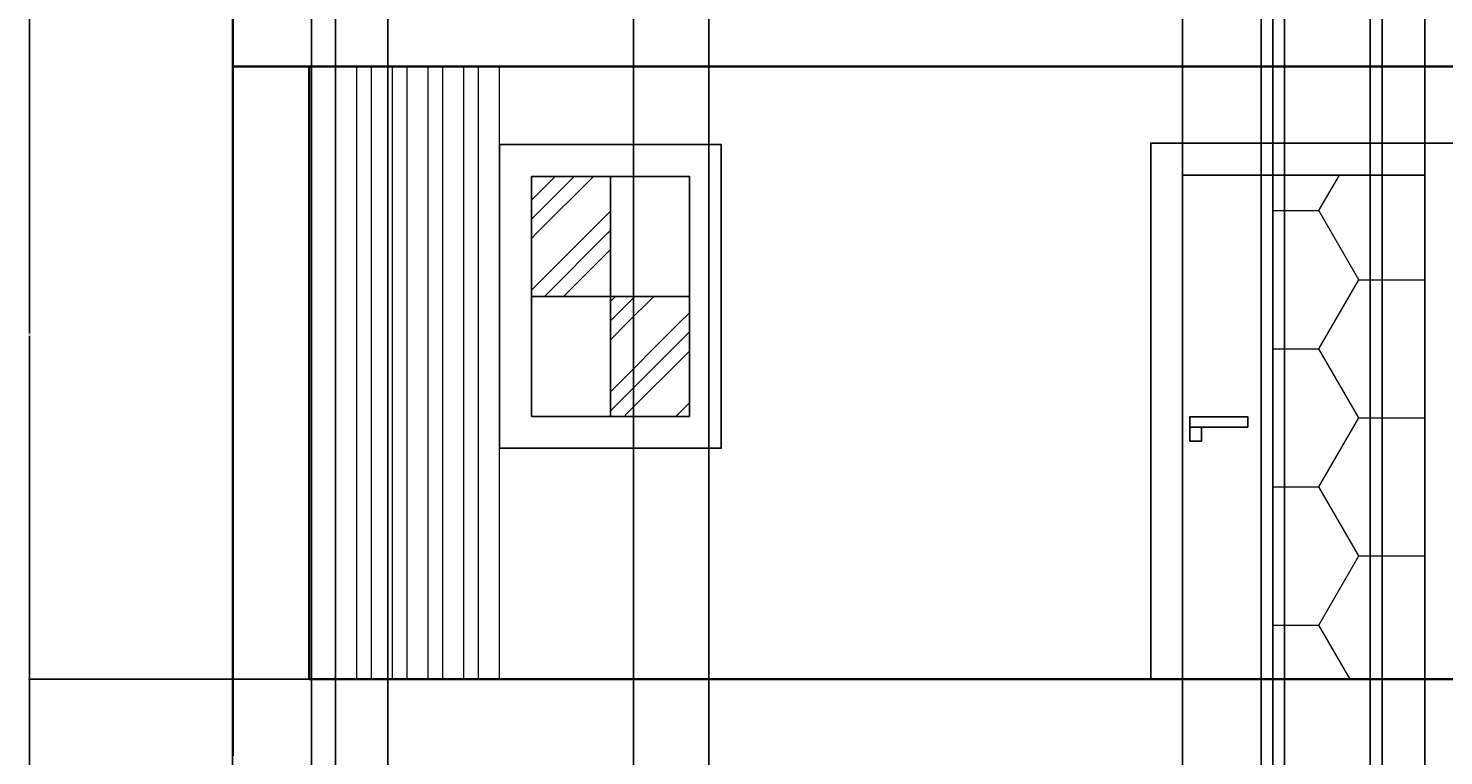
# Model space of a CAD drawing. Units: inches. Extents: x -8 to 554, y -200 to 499.
# Tile 2 of 12: x -8 to 214, y 7 to 121. Entities that reach past the tile are written whole.
import ezdxf

# ---------------------------------------------------------------- set-up
doc = ezdxf.new("R2010")
doc.units = ezdxf.units.IN
doc.header["$MEASUREMENT"] = 0
for name, color, linetype, lineweight in [('A-ANNO-DIMS', 2, 'Continuous', 18), ('A-DOOR', 3, 'Continuous', 25), ('A-DOOR-PATT', 252, 'Continuous', 13), ('A-FLOR', 7, 'Continuous', 35), ('A-GLAZ', 4, 'Continuous', 25), ('A-GLAZ-PATT', 252, 'Continuous', 13), ('A-WALL', 7, 'Continuous', 35), ('A-WALL-SCRN', 8, 'Continuous', 18)]:
    doc.layers.add(name, color=color, linetype=linetype, lineweight=lineweight)
doc.styles.get("Standard").update_dxf_attribs({"font": 'arial.ttf'})
doc.dimstyles.get("Standard").update_dxf_attribs({"dimtxt": 0.18, "dimasz": 0.18, "dimexe": 0.18, "dimexo": 0.0625, "dimgap": 0.09, "dimtad": 0, "dimtih": 1, "dimtoh": 1, "dimdec": 4, "dimzin": 0, "dimdsep": 46, "dimtxsty": 'Standard', "dimcen": 0.09, "dimadec": 0, "dimazin": 0, "dimtfac": 1, "dimtdec": 4, "dimtofl": 0, "dimtmove": 0, "dimatfit": 3, "dimfxl": 1, "dimtolj": 1, "dimtzin": 0, "dimarcsym": 0})

# ---------------------------------------------------------------- blocks, each defined once
blk = doc.blocks.new('DOOR-LEVER-ELEV')
for points in [[(0, 2.19), (9.08, 2.19), (9.08, 3.81), (0, 3.81)], [(0, 2.19), (1.8, 2.19), (1.8, 0), (0, 0)]]:
    blk.add_lwpolyline(points, close=True)
blk = doc.blocks.new('SCREEN-FIVE-FINS-ELEV')
for points in [[(0, 0), (3.37, 0), (3.37, 96), (0, 96)], [(5.59, 0), (8.97, 0), (8.97, 96), (5.59, 96)], [(11.19, 0), (14.56, 0), (14.56, 96), (11.19, 96)], [(16.78, 0), (20.16, 0), (20.16, 96), (16.78, 96)], [(22.38, 0), (25.75, 0), (25.75, 96), (22.38, 96)]]:
    blk.add_lwpolyline(points, close=True)
blk = doc.blocks.new('WINDOW-CASING-FOUR-LIGHT')
blk.add_lwpolyline([(0, 47.61), (34.77, 47.61), (34.77, 0), (0, 0)], close=True)
blk = doc.blocks.new('*D31')
at = {"layer": 'A-ANNO-DIMS', "color": 0, "lineweight": -2, "transparency": 16777216}
for p, q in [((24.34, 127.42), (24.34, -199.97)), ((453.32, -30.73), (453.32, -199.97)), ((24.52, -199.79), (238.54, -199.79)), ((453.14, -199.79), (239.12, -199.79))]:
    blk.add_line(p, q, dxfattribs=at)
at = {"layer": 'A-ANNO-DIMS', "color": 0, "transparency": 16777216}
for points in [[(24.52, -199.76), (24.52, -199.82), (24.34, -199.79)], [(453.14, -199.76), (453.14, -199.82), (453.32, -199.79)]]:
    blk.add_solid(points, dxfattribs=at)
at = {"layer": 'Defpoints', "color": 0, "transparency": 16777216}
for p in [(24.34, 127.48), (453.32, -30.67), (453.32, -199.79)]:
    blk.add_point(p, dxfattribs=at)
at = {"layer": 'A-ANNO-DIMS', "color": 0, "transparency": 16777216, "insert": (238.83, -199.79), "char_height": 0.18, "attachment_point": 5}
blk.add_mtext('\\A1;429', dxfattribs=at)
blk = doc.blocks.new('*D32')
at = {"layer": 'A-ANNO-DIMS', "color": 0, "lineweight": -2, "transparency": 16777216}
for p, q in [((24.34, 223.42), (24.34, -199.97)), ((444.34, 223.42), (444.34, -199.97)), ((24.52, -199.79), (234.05, -199.79)), ((444.16, -199.79), (234.63, -199.79))]:
    blk.add_line(p, q, dxfattribs=at)
at = {"layer": 'A-ANNO-DIMS', "color": 0, "transparency": 16777216}
for points in [[(24.52, -199.76), (24.52, -199.82), (24.34, -199.79)], [(444.16, -199.76), (444.16, -199.82), (444.34, -199.79)]]:
    blk.add_solid(points, dxfattribs=at)
at = {"layer": 'Defpoints', "color": 0, "transparency": 16777216}
for p in [(24.34, 223.48), (444.34, 223.48), (444.34, -199.79)]:
    blk.add_point(p, dxfattribs=at)
at = {"layer": 'A-ANNO-DIMS', "color": 0, "transparency": 16777216, "insert": (234.34, -199.79), "char_height": 0.18, "attachment_point": 5}
blk.add_mtext('\\A1;420', dxfattribs=at)
blk = doc.blocks.new('*D33')
at = {"layer": 'A-ANNO-DIMS', "color": 0, "lineweight": -2, "transparency": 16777216}
for p, q in [((36.28, 19.48), (-7.69, 19.48)), ((-7.51, 19.3), (-7.51, -46.34)), ((-7.51, -112.34), (-7.51, -46.7)), ((24.28, -112.52), (-7.69, -112.52))]:
    blk.add_line(p, q, dxfattribs=at)
at = {"layer": 'A-ANNO-DIMS', "color": 0, "transparency": 16777216}
for points in [[(-7.54, 19.3), (-7.48, 19.3), (-7.51, 19.48)], [(-7.54, -112.34), (-7.48, -112.34), (-7.51, -112.52)]]:
    blk.add_solid(points, dxfattribs=at)
at = {"layer": 'Defpoints', "color": 0, "transparency": 16777216}
for p in [(-7.51, 19.48), (36.34, 19.48), (24.34, -112.52)]:
    blk.add_point(p, dxfattribs=at)
at = {"layer": 'A-ANNO-DIMS', "color": 0, "transparency": 16777216, "insert": (-7.51, -46.52), "char_height": 0.18, "attachment_point": 5}
blk.add_mtext('\\A1;132', dxfattribs=at)
blk = doc.blocks.new('*D34')
at = {"layer": 'A-ANNO-DIMS', "color": 0, "lineweight": -2, "transparency": 16777216}
for p, q in [((24.28, 127.48), (-7.69, 127.48)), ((-7.51, 127.3), (-7.51, 73.66)), ((-7.51, 19.66), (-7.51, 73.3)), ((36.28, 19.48), (-7.69, 19.48))]:
    blk.add_line(p, q, dxfattribs=at)
at = {"layer": 'A-ANNO-DIMS', "color": 0, "transparency": 16777216}
for points in [[(-7.54, 127.3), (-7.48, 127.3), (-7.51, 127.48)], [(-7.54, 19.66), (-7.48, 19.66), (-7.51, 19.48)]]:
    blk.add_solid(points, dxfattribs=at)
at = {"layer": 'Defpoints', "color": 0, "transparency": 16777216}
for p in [(-7.51, 127.48), (24.34, 127.48), (36.34, 19.48)]:
    blk.add_point(p, dxfattribs=at)
at = {"layer": 'A-ANNO-DIMS', "color": 0, "transparency": 16777216, "insert": (-7.51, 73.48), "char_height": 0.18, "attachment_point": 5}
blk.add_mtext('\\A1;108', dxfattribs=at)
blk = doc.blocks.new('*D41')
at = {"layer": 'A-ANNO-DIMS', "color": 0, "lineweight": -2, "transparency": 16777216}
for p, q in [((24.34, 235.42), (24.34, -199.97)), ((40.45, 235.42), (40.45, -199.97)), ((24.52, -199.79), (31.94, -199.79)), ((40.27, -199.79), (32.85, -199.79))]:
    blk.add_line(p, q, dxfattribs=at)
at = {"layer": 'A-ANNO-DIMS', "color": 0, "transparency": 16777216}
for points in [[(24.52, -199.76), (24.52, -199.82), (24.34, -199.79)], [(40.27, -199.76), (40.27, -199.82), (40.45, -199.79)]]:
    blk.add_solid(points, dxfattribs=at)
at = {"layer": 'Defpoints', "color": 0, "transparency": 16777216}
for p in [(24.34, 235.48), (40.45, 235.48), (40.45, -199.79)]:
    blk.add_point(p, dxfattribs=at)
at = {"layer": 'A-ANNO-DIMS', "color": 0, "transparency": 16777216, "insert": (32.4, -199.79), "char_height": 0.18, "attachment_point": 5}
blk.add_mtext('\\A1;16.113', dxfattribs=at)
blk = doc.blocks.new('*D55')
at = {"layer": 'A-ANNO-DIMS', "color": 0, "lineweight": -2, "transparency": 16777216}
for p, q in [((204.61, -30.61), (204.61, 498.99)), ((204.79, 498.81), (328.57, 498.81)), ((453.14, 498.81), (329.36, 498.81)), ((453.32, -30.61), (453.32, 498.99))]:
    blk.add_line(p, q, dxfattribs=at)
at = {"layer": 'A-ANNO-DIMS', "color": 0, "transparency": 16777216}
for points in [[(204.79, 498.84), (204.79, 498.78), (204.61, 498.81)], [(453.14, 498.84), (453.14, 498.78), (453.32, 498.81)]]:
    blk.add_solid(points, dxfattribs=at)
at = {"layer": 'Defpoints', "color": 0, "transparency": 16777216}
for p in [(453.32, 498.81), (204.61, -30.67), (453.32, -30.67)]:
    blk.add_point(p, dxfattribs=at)
at = {"layer": 'A-ANNO-DIMS', "color": 0, "transparency": 16777216, "insert": (328.96, 498.81), "char_height": 0.18, "attachment_point": 5}
blk.add_mtext('\\A1;248.7', dxfattribs=at)
blk = doc.blocks.new('*D56')
at = {"layer": 'A-ANNO-DIMS', "color": 0, "lineweight": -2, "transparency": 16777216}
for p, q in [((24.34, 7.54), (24.34, 498.99)), ((24.52, 498.81), (30.06, 498.81)), ((36.51, 498.81), (30.97, 498.81)), ((36.69, 7.54), (36.69, 498.99))]:
    blk.add_line(p, q, dxfattribs=at)
at = {"layer": 'A-ANNO-DIMS', "color": 0, "transparency": 16777216}
for points in [[(24.52, 498.84), (24.52, 498.78), (24.34, 498.81)], [(36.51, 498.84), (36.51, 498.78), (36.69, 498.81)]]:
    blk.add_solid(points, dxfattribs=at)
at = {"layer": 'Defpoints', "color": 0, "transparency": 16777216}
for p in [(36.69, 498.81), (24.34, 7.48), (36.69, 7.48)]:
    blk.add_point(p, dxfattribs=at)
at = {"layer": 'A-ANNO-DIMS', "color": 0, "transparency": 16777216, "insert": (30.52, 498.81), "char_height": 0.18, "attachment_point": 5}
blk.add_mtext('\\A1;12.346', dxfattribs=at)
blk = doc.blocks.new('*D57')
at = {"layer": 'A-ANNO-DIMS', "color": 0, "lineweight": -2, "transparency": 16777216}
for p, q in [((36.69, -52.46), (36.69, 498.99)), ((36.87, 498.81), (42.48, 498.81)), ((48.51, 498.81), (42.9, 498.81)), ((48.69, -52.46), (48.69, 498.99))]:
    blk.add_line(p, q, dxfattribs=at)
at = {"layer": 'A-ANNO-DIMS', "color": 0, "transparency": 16777216}
for points in [[(36.87, 498.84), (36.87, 498.78), (36.69, 498.81)], [(48.51, 498.84), (48.51, 498.78), (48.69, 498.81)]]:
    blk.add_solid(points, dxfattribs=at)
at = {"layer": 'Defpoints', "color": 0, "transparency": 16777216}
for p in [(48.69, 498.81), (36.69, -52.52), (48.69, -52.52)]:
    blk.add_point(p, dxfattribs=at)
at = {"layer": 'A-ANNO-DIMS', "color": 0, "transparency": 16777216, "insert": (42.69, 498.81), "char_height": 0.18, "attachment_point": 5}
blk.add_mtext('\\A1;12', dxfattribs=at)
blk = doc.blocks.new('*D58')
at = {"layer": 'A-ANNO-DIMS', "color": 0, "lineweight": -2, "transparency": 16777216}
for p, q in [((36.69, 7.54), (36.69, 498.99)), ((36.87, 498.81), (61.56, 498.81)), ((87.03, 498.81), (62.34, 498.81)), ((87.21, 7.54), (87.21, 498.99))]:
    blk.add_line(p, q, dxfattribs=at)
at = {"layer": 'A-ANNO-DIMS', "color": 0, "transparency": 16777216}
for points in [[(36.87, 498.84), (36.87, 498.78), (36.69, 498.81)], [(87.03, 498.84), (87.03, 498.78), (87.21, 498.81)]]:
    blk.add_solid(points, dxfattribs=at)
at = {"layer": 'Defpoints', "color": 0, "transparency": 16777216}
for p in [(87.21, 498.81), (36.69, 7.48), (87.21, 7.48)]:
    blk.add_point(p, dxfattribs=at)
at = {"layer": 'A-ANNO-DIMS', "color": 0, "transparency": 16777216, "insert": (61.95, 498.81), "char_height": 0.18, "attachment_point": 5}
blk.add_mtext('\\A1;50.52', dxfattribs=at)
blk = doc.blocks.new('*D59')
at = {"layer": 'A-ANNO-DIMS', "color": 0, "lineweight": -2, "transparency": 16777216}
for p, q in [((87.21, -60.84), (87.21, 498.99)), ((87.39, 498.81), (92.67, 498.81)), ((98.86, 498.81), (93.58, 498.81)), ((99.04, -60.84), (99.04, 498.99))]:
    blk.add_line(p, q, dxfattribs=at)
at = {"layer": 'A-ANNO-DIMS', "color": 0, "transparency": 16777216}
for points in [[(87.39, 498.84), (87.39, 498.78), (87.21, 498.81)], [(98.86, 498.84), (98.86, 498.78), (99.04, 498.81)]]:
    blk.add_solid(points, dxfattribs=at)
at = {"layer": 'Defpoints', "color": 0, "transparency": 16777216}
for p in [(99.04, 498.81), (87.21, -60.9), (99.04, -60.9)]:
    blk.add_point(p, dxfattribs=at)
at = {"layer": 'A-ANNO-DIMS', "color": 0, "transparency": 16777216, "insert": (93.12, 498.81), "char_height": 0.18, "attachment_point": 5}
blk.add_mtext('\\A1;11.827', dxfattribs=at)
blk = doc.blocks.new('*D60')
at = {"layer": 'A-ANNO-DIMS', "color": 0, "lineweight": -2, "transparency": 16777216}
for p, q in [((87.21, 7.54), (87.21, 498.99)), ((87.39, 498.81), (137.89, 498.81)), ((189.12, 498.81), (138.63, 498.81)), ((189.3, 7.54), (189.3, 498.99))]:
    blk.add_line(p, q, dxfattribs=at)
at = {"layer": 'A-ANNO-DIMS', "color": 0, "transparency": 16777216}
for points in [[(87.39, 498.84), (87.39, 498.78), (87.21, 498.81)], [(189.12, 498.84), (189.12, 498.78), (189.3, 498.81)]]:
    blk.add_solid(points, dxfattribs=at)
at = {"layer": 'Defpoints', "color": 0, "transparency": 16777216}
for p in [(189.3, 498.81), (87.21, 7.48), (189.3, 7.48)]:
    blk.add_point(p, dxfattribs=at)
at = {"layer": 'A-ANNO-DIMS', "color": 0, "transparency": 16777216, "insert": (138.26, 498.81), "char_height": 0.18, "attachment_point": 5}
blk.add_mtext('\\A1;102.1', dxfattribs=at)
blk = doc.blocks.new('*D61')
at = {"layer": 'A-ANNO-DIMS', "color": 0, "lineweight": -2, "transparency": 16777216}
for p, q in [((189.3, -52.46), (189.3, 498.99)), ((189.48, 498.81), (195.57, 498.81)), ((202.57, 498.81), (196.48, 498.81)), ((202.75, -52.46), (202.75, 498.99))]:
    blk.add_line(p, q, dxfattribs=at)
at = {"layer": 'A-ANNO-DIMS', "color": 0, "transparency": 16777216}
for points in [[(189.48, 498.84), (189.48, 498.78), (189.3, 498.81)], [(202.57, 498.84), (202.57, 498.78), (202.75, 498.81)]]:
    blk.add_solid(points, dxfattribs=at)
at = {"layer": 'Defpoints', "color": 0, "transparency": 16777216}
for p in [(202.75, 498.81), (189.3, -52.52), (202.75, -52.52)]:
    blk.add_point(p, dxfattribs=at)
at = {"layer": 'A-ANNO-DIMS', "color": 0, "transparency": 16777216, "insert": (196.03, 498.81), "char_height": 0.18, "attachment_point": 5}
blk.add_mtext('\\A1;13.446', dxfattribs=at)
blk = doc.blocks.new('*D62')
at = {"layer": 'A-ANNO-DIMS', "color": 0, "lineweight": -2, "transparency": 16777216}
for p, q in [((189.3, 7.54), (189.3, 498.99)), ((189.48, 498.81), (263.01, 498.81)), ((337.31, 498.81), (263.78, 498.81)), ((337.49, 7.54), (337.49, 498.99))]:
    blk.add_line(p, q, dxfattribs=at)
at = {"layer": 'A-ANNO-DIMS', "color": 0, "transparency": 16777216}
for points in [[(189.48, 498.84), (189.48, 498.78), (189.3, 498.81)], [(337.31, 498.84), (337.31, 498.78), (337.49, 498.81)]]:
    blk.add_solid(points, dxfattribs=at)
at = {"layer": 'Defpoints', "color": 0, "transparency": 16777216}
for p in [(337.49, 498.81), (189.3, 7.48), (337.49, 7.48)]:
    blk.add_point(p, dxfattribs=at)
at = {"layer": 'A-ANNO-DIMS', "color": 0, "transparency": 16777216, "insert": (263.4, 498.81), "char_height": 0.18, "attachment_point": 5}
blk.add_mtext('\\A1;148.2', dxfattribs=at)
blk = doc.blocks.new('*D80')
at = {"layer": 'A-ANNO-DIMS', "color": 0, "lineweight": -2, "transparency": 16777216}
for p, q in [((173.34, 314.42), (173.34, -199.97)), ((211.34, 314.42), (211.34, -199.97)), ((173.52, -199.79), (192.12, -199.79)), ((211.16, -199.79), (192.56, -199.79))]:
    blk.add_line(p, q, dxfattribs=at)
at = {"layer": 'A-ANNO-DIMS', "color": 0, "transparency": 16777216}
for points in [[(173.52, -199.76), (173.52, -199.82), (173.34, -199.79)], [(211.16, -199.76), (211.16, -199.82), (211.34, -199.79)]]:
    blk.add_solid(points, dxfattribs=at)
at = {"layer": 'Defpoints', "color": 0, "transparency": 16777216}
for p in [(173.34, 314.48), (211.34, 314.48), (211.34, -199.79)]:
    blk.add_point(p, dxfattribs=at)
at = {"layer": 'A-ANNO-DIMS', "color": 0, "transparency": 16777216, "insert": (192.34, -199.79), "char_height": 0.18, "attachment_point": 5}
blk.add_mtext('\\A1;38', dxfattribs=at)
blk = doc.blocks.new('*D81')
at = {"layer": 'A-ANNO-DIMS', "color": 0, "lineweight": -2, "transparency": 16777216}
for p, q in [((173.34, 235.42), (173.34, -199.97)), ((185.64, 235.42), (185.64, -199.97)), ((173.52, -199.79), (179.04, -199.79)), ((185.46, -199.79), (179.95, -199.79))]:
    blk.add_line(p, q, dxfattribs=at)
at = {"layer": 'A-ANNO-DIMS', "color": 0, "transparency": 16777216}
for points in [[(173.52, -199.76), (173.52, -199.82), (173.34, -199.79)], [(185.46, -199.76), (185.46, -199.82), (185.64, -199.79)]]:
    blk.add_solid(points, dxfattribs=at)
at = {"layer": 'Defpoints', "color": 0, "transparency": 16777216}
for p in [(173.34, 235.48), (185.64, 235.48), (185.64, -199.79)]:
    blk.add_point(p, dxfattribs=at)
at = {"layer": 'A-ANNO-DIMS', "color": 0, "transparency": 16777216, "insert": (179.49, -199.79), "char_height": 0.18, "attachment_point": 5}
blk.add_mtext('\\A1;12.302', dxfattribs=at)
blk = doc.blocks.new('*D82')
at = {"layer": 'A-ANNO-DIMS', "color": 0, "lineweight": -2, "transparency": 16777216}
for p, q in [((185.64, 235.42), (185.64, -199.97)), ((187.48, 235.42), (187.48, -199.97)), ((185.82, -199.79), (186.18, -199.79)), ((187.3, -199.79), (186.95, -199.79))]:
    blk.add_line(p, q, dxfattribs=at)
at = {"layer": 'A-ANNO-DIMS', "color": 0, "transparency": 16777216}
for points in [[(185.82, -199.76), (185.82, -199.82), (185.64, -199.79)], [(187.3, -199.76), (187.3, -199.82), (187.48, -199.79)]]:
    blk.add_solid(points, dxfattribs=at)
at = {"layer": 'Defpoints', "color": 0, "transparency": 16777216}
for p in [(185.64, 235.48), (187.48, 235.48), (187.48, -199.79)]:
    blk.add_point(p, dxfattribs=at)
at = {"layer": 'A-ANNO-DIMS', "color": 0, "transparency": 16777216, "insert": (186.56, -199.79), "char_height": 0.18, "attachment_point": 5}
blk.add_mtext('\\A1;1.837', dxfattribs=at)

msp = doc.modelspace()

# ---------------------------------------------------------------- hatches: boundary and pattern name
at = {"layer": 'A-DOOR-PATT', "transparency": 33554523}
h = msp.add_hatch(dxfattribs=at)
h.set_pattern_fill('HONEY', color=256, scale=100)
h.set_pattern_definition([(0, (-117.809, -80.312), (18.75, 10.82532), [12.5, -25]), (120, (-117.809, -80.312), (-18.75, 10.82532), [12.5, -25]), (60, (-117.809, -80.312), (4e-15, 21.65064), [-25, 12.5])])
h.paths.add_polyline_path([(211.3421, 314.4814), (187.4809, 314.4814), (187.4809, 235.4814), (211.3421, 235.4814)])
h.paths.add_polyline_path([(211.3421, 206.4814), (187.4809, 206.4814), (187.4809, 127.4814), (211.3421, 127.4814)])
h.paths.add_polyline_path([(211.3421, 98.4814), (187.4809, 98.4814), (187.4809, 19.4814), (211.3421, 19.4814)])
h.paths.add_polyline_path([(432.5174, 98.4814), (408.6562, 98.4814), (408.6562, 19.4814), (432.5174, 19.4814)])
h.paths.add_polyline_path([(432.5174, 206.4814), (408.6562, 206.4814), (408.6562, 127.4814), (432.5174, 127.4814), (432.5174, 155.7921)])
h.paths.add_polyline_path([(432.5174, 314.4814), (408.6562, 314.4814), (408.6562, 235.4814), (432.5174, 235.4814)])
at = {"layer": 'A-GLAZ-PATT'}
h = msp.add_hatch(dxfattribs=at)
h.set_pattern_fill('GOST_GROUND', color=256)
h.set_pattern_definition([(45, (-117.809, -80.312), (14.14214, 0), [20]), (45, (-114.809, -80.312), (14.14214, 0), [20]), (45, (-111.809, -80.312), (14.14214, 0), [20])])
h.paths.add_polyline_path([(83.5906, 206.2713), (71.2048, 206.2713), (71.2048, 187.4661), (83.5906, 187.4661)])
h.paths.add_polyline_path([(95.9765, 187.4661), (83.5906, 187.4661), (83.5906, 168.661), (95.9765, 168.661)])
h.paths.add_polyline_path([(83.5906, 98.2713), (71.2048, 98.2713), (71.2048, 79.4661), (83.5906, 79.4661)])
h.paths.add_polyline_path([(95.9765, 79.4661), (83.5906, 79.4661), (83.5906, 60.661), (95.9765, 60.661)])
h.paths.add_polyline_path([(333.2924, 98.788), (317.3421, 98.788), (317.3421, 61.7623), (333.2924, 61.7623)])
h.paths.add_polyline_path([(352.699, 98.788), (336.6386, 98.788), (336.6386, 61.7623), (352.699, 61.7623)])
h.paths.add_polyline_path([(333.2924, 206.788), (317.3421, 206.788), (317.3421, 169.7623), (333.2924, 169.7623)])
h.paths.add_polyline_path([(352.699, 206.788), (336.6386, 206.788), (336.6386, 169.7623), (352.699, 169.7623)])
h.paths.add_polyline_path([(333.2924, 314.788), (317.3421, 314.788), (317.3421, 277.7623), (333.2924, 277.7623)])
h.paths.add_polyline_path([(352.699, 314.788), (336.6386, 314.788), (336.6386, 277.7623), (352.699, 277.7623)])
h.paths.add_polyline_path([(95.9765, 295.4661), (83.5906, 295.4661), (83.5906, 276.661), (95.9765, 276.661)])
h.paths.add_polyline_path([(83.5906, 314.2713), (71.2048, 314.2713), (71.2048, 295.4661), (83.5906, 295.4661)])

# ---------------------------------------------------------------- linework, layer by layer
at = {"layer": 'A-DOOR'}
for p, q in [((173.3421, 19.4814), (173.3421, 98.4814)), ((173.3421, 98.4814), (211.3421, 98.4814)), ((211.3421, 98.4814), (211.3421, 19.4814))]:
    msp.add_line(p, q, dxfattribs=at)
for points in [[(216.3421, 19.4814), (168.3421, 19.4814), (168.3421, 103.4814), (216.3421, 103.4814)], [(185.644, 98.4814), (187.4809, 98.4814), (187.4809, 19.4814), (185.644, 19.4814)]]:
    msp.add_lwpolyline(points, close=True, dxfattribs=at)
at = {"layer": 'A-FLOR'}
for p, q in [((24.3421, 115.4814), (444.3421, 115.4814)), ((444.3421, 115.4814), (36.3421, 115.4814)), ((36.3421, 19.4814), (444.3421, 19.4814))]:
    msp.add_line(p, q, dxfattribs=at)
at = {"layer": 'A-GLAZ'}
for p, q in [((83.5906, 98.2713), (83.5906, 60.661)), ((71.2048, 79.4661), (95.9765, 79.4661))]:
    msp.add_line(p, q, dxfattribs=at)
msp.add_lwpolyline([(71.2048, 98.2713), (95.9765, 98.2713), (95.9765, 60.661), (71.2048, 60.661)], close=True, dxfattribs=at)
at = {"layer": 'A-WALL'}
for p, q in [((24.3421, 235.4814), (24.3421, 115.4814)), ((24.3421, 127.4814), (24.3421, 7.4814)), ((36.3421, 115.4814), (36.3421, 19.4814))]:
    msp.add_line(p, q, dxfattribs=at)

# ---------------------------------------------------------------- block references
at = {"layer": 'A-DOOR'}
msp.add_blockref('DOOR-LEVER-ELEV', (174.4762, 56.7884), dxfattribs=at)
at = {"layer": 'A-GLAZ'}
msp.add_blockref('WINDOW-CASING-FOUR-LIGHT', (66.2048, 55.661), dxfattribs=at)
at = {"layer": 'A-WALL-SCRN'}
msp.add_blockref('SCREEN-FIVE-FINS-ELEV', (40.4549, 19.4814), dxfattribs=at)

# ---------------------------------------------------------------- dimensions: what is measured, and where the dimension line sits
at = {"layer": 'A-ANNO-DIMS'}
for base, p1, p2, override, picture, middle in [((36.6882, 498.8091), (24.3421, 7.4814), (36.6882, 7.4814), {"dimdec": 3, "dimlfac": 1, "dimrnd": 0, "dimzin": 0, "dimdsep": 46, "dimlunit": 2}, '*D56', (30.5151, 498.8091)), ((48.6882, 498.8091), (36.6882, -52.5186), (48.6882, -52.5186), {"dimdec": 0, "dimlfac": 1, "dimrnd": 0, "dimzin": 0, "dimdsep": 46, "dimlunit": 2}, '*D57', (42.6882, 498.8091)), ((87.21, 498.8091), (36.6882, 7.4814), (87.21, 7.4814), {"dimdec": 2, "dimlfac": 1, "dimrnd": 0, "dimzin": 0, "dimdsep": 46, "dimlunit": 2}, '*D58', (61.9491, 498.8091)), ((99.037, 498.8091), (87.21, -60.9032), (99.037, -60.9032), {"dimdec": 3, "dimlfac": 1, "dimrnd": 0, "dimzin": 0, "dimdsep": 46, "dimlunit": 2}, '*D59', (93.1235, 498.8091)), ((189.3049, 498.8091), (87.21, 7.4814), (189.3049, 7.4814), {"dimdec": 1, "dimlfac": 1, "dimrnd": 0, "dimzin": 0, "dimdsep": 46, "dimlunit": 2}, '*D60', (138.2575, 498.8091)), ((202.7513, 498.8091), (189.3049, -52.5186), (202.7513, -52.5186), {"dimdec": 3, "dimlfac": 1, "dimrnd": 0, "dimzin": 0, "dimdsep": 46, "dimlunit": 2}, '*D61', (196.0281, 498.8091)), ((337.4923, 498.8091), (189.3049, 7.4814), (337.4923, 7.4814), {"dimdec": 1, "dimlfac": 1, "dimrnd": 0, "dimzin": 0, "dimdsep": 46, "dimlunit": 2}, '*D62', (263.3986, 498.8091)), ((453.3222, 498.8091), (204.6055, -30.6677), (453.3222, -30.6677), {"dimdec": 1, "dimlfac": 1, "dimrnd": 0, "dimzin": 0, "dimdsep": 46, "dimlunit": 2}, '*D55', (328.9639, 498.8091)), ((211.3421, -199.7912), (173.3421, 314.4814), (211.3421, 314.4814), {"dimdec": 0, "dimlfac": 1, "dimrnd": 0, "dimzin": 0, "dimdsep": 46, "dimlunit": 2}, '*D80', (192.3421, -199.7912)), ((40.4549, -199.7912), (24.3421, 235.4814), (40.4549, 235.4814), {"dimdec": 3, "dimlfac": 1, "dimrnd": 0, "dimzin": 0, "dimdsep": 46, "dimlunit": 2}, '*D41', (32.3985, -199.7912)), ((185.644, -199.7912), (173.3421, 235.4814), (185.644, 235.4814), {"dimdec": 3, "dimlfac": 1, "dimrnd": 0, "dimzin": 0, "dimdsep": 46, "dimlunit": 2}, '*D81', (179.493, -199.7912)), ((187.4809, -199.7912), (185.644, 235.4814), (187.4809, 235.4814), {"dimdec": 3, "dimlfac": 1, "dimrnd": 0, "dimzin": 0, "dimdsep": 46, "dimlunit": 2}, '*D82', (186.5625, -199.7912)), ((444.3421, -199.7912), (24.3421, 223.4814), (444.3421, 223.4814), {"dimdec": 0, "dimlfac": 1, "dimrnd": 0, "dimzin": 0, "dimdsep": 46, "dimlunit": 2}, '*D32', (234.3421, -199.7912)), ((453.3222, -199.7912), (24.3421, 127.4814), (453.3222, -30.6677), {"dimdec": 0, "dimlfac": 1, "dimrnd": 0, "dimzin": 0, "dimdsep": 46, "dimlunit": 2}, '*D31', (238.8321, -199.7912))]:
    dim = msp.add_linear_dim(base=base, p1=p1, p2=p2, dimstyle='Standard', override=override, dxfattribs=at)
    dim.commit()
    dim.dimension.update_dxf_attribs({"geometry": picture, "text_midpoint": middle})
for base, p1, p2, picture, middle in [((-7.5079, 127.4814), (36.3421, 19.4814), (24.3421, 127.4814), '*D34', (-7.5079, 73.4814)), ((-7.5079, 19.4814), (24.3421, -112.5186), (36.3421, 19.4814), '*D33', (-7.5079, -46.5186))]:
    dim = msp.add_linear_dim(base=base, p1=p1, p2=p2, angle=90, dimstyle='Standard', override={"dimdec": 0, "dimlfac": 1, "dimrnd": 0, "dimzin": 0, "dimdsep": 46, "dimlunit": 2}, dxfattribs=at)
    dim.commit()
    dim.dimension.update_dxf_attribs({"geometry": picture, "text_midpoint": middle})

doc.saveas('drawing.dxf')
